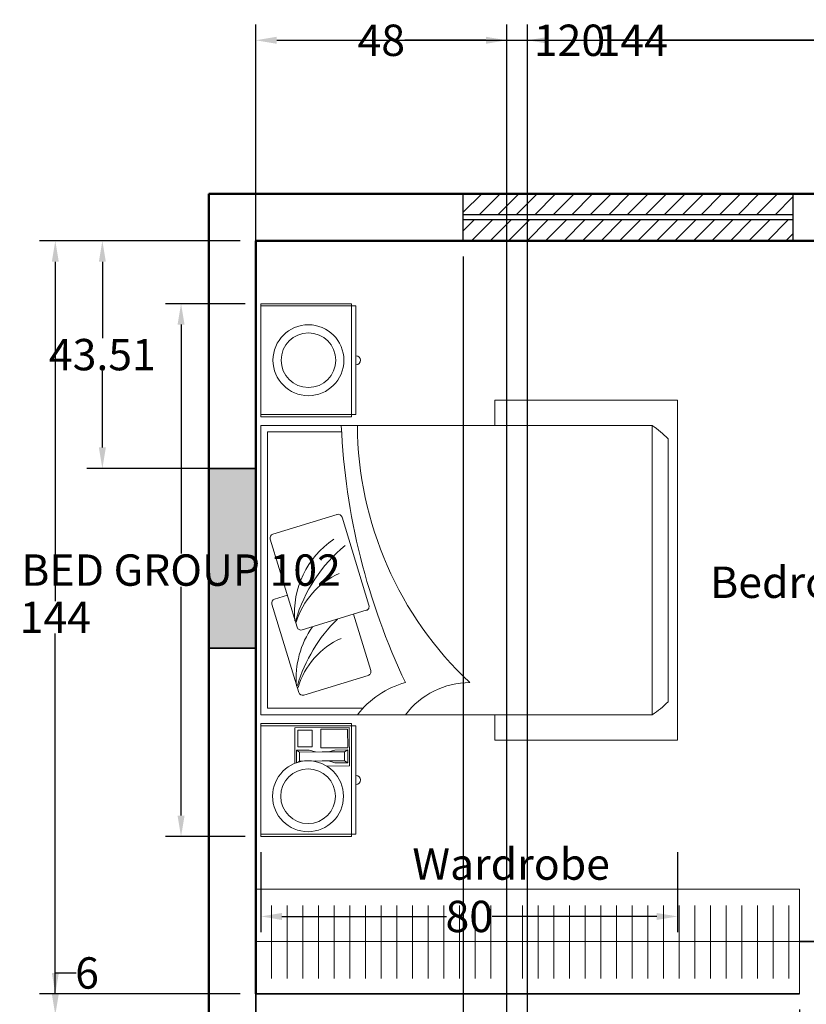
# Model space of a CAD drawing. Units: inches. Extents: x -1285 to -837, y -84 to 552.
# Tile 6 of 10: x -1282 to -1131, y 364 to 552. Entities that reach past the tile are written whole.
import ezdxf

# ---------------------------------------------------------------- set-up
doc = ezdxf.new("R2010")
doc.units = ezdxf.units.IN
doc.header["$MEASUREMENT"] = 0
for name, color, linetype, lineweight in [('A-ANNO-DIMS', 2, 'Continuous', 18), ('A-ANNO-TEXT', 7, 'Continuous', 18), ('A-AREA-IDEN', 7, 'Continuous', 25), ('A-COLS', 54, 'Continuous', 35), ('A-COLS-PATT', 54, 'Continuous', 13), ('A-GLAZ-PATT', 191, 'Continuous', 13), ('Beds', 74, 'Continuous', 18), ('Inner Wall', 202, 'Continuous', 35), ('Outer Wall', 12, 'Continuous', 50), ('Wardrobe', 145, 'Continuous', 18), ('Windows', 191, 'Continuous', 25)]:
    doc.layers.add(name, color=color, linetype=linetype, lineweight=lineweight)
doc.styles.get("Standard").update_dxf_attribs({"font": 'arial.ttf'})
doc.dimstyles.get("Standard").update_dxf_attribs({"dimtxt": 6, "dimasz": 4, "dimexe": 3, "dimexo": 3, "dimgap": 0.09, "dimtad": 0, "dimtih": 1, "dimtoh": 1, "dimdec": 1, "dimzin": 0, "dimdsep": 46, "dimlunit": 3, "dimtxsty": 'Standard', "dimcen": 0.09, "dimadec": 0, "dimazin": 0, "dimtfac": 1, "dimtdec": 1, "dimtofl": 0, "dimtmove": 0, "dimatfit": 3, "dimfxl": 1, "dimtolj": 1, "dimtzin": 0, "dimarcsym": 0})

# ---------------------------------------------------------------- blocks, each defined once
blk = doc.blocks.new('Double bed')
for p, q in [((1422.016, 1006.492), (1422.016, 1015.393)), ((1422.016, 1015.393), (1433.142, 1015.393)), ((1422.239, 1006.047), (1422.239, 1015.393)), ((1432.92, 1015.393), (1432.92, 1006.047)), ((1433.142, 1015.393), (1433.142, 1006.492)), ((1433.999, 1015.393), (1433.999, 1005.908)), ((1462.453, 1015.393), (1433.999, 1015.393)), ((1462.453, 1007.489), (1462.453, 1015.393)), ((1463.309, 1015.393), (1463.309, 1006.491)), ((1474.436, 1015.393), (1463.309, 1015.393)), ((1463.531, 1015.393), (1463.531, 1006.046)), ((1474.214, 1006.046), (1474.214, 1015.393)), ((1474.436, 1006.491), (1474.436, 1015.393)), ((1444.87, 1014.313), (1436.198, 1011.659)), ((1451.273, 1014.487), (1442.6, 1011.833)), ((1451.766, 1014.225), (1453.699, 1007.909)), ((1445.364, 1014.05), (1445.748, 1012.796)), ((1432.723, 1012.072), (1429.217, 1012.059)), ((1429.252, 1011.901), (1430.515, 1011.906)), ((1429.443, 1011.586), (1429.252, 1011.901)), ((1429.443, 1011.586), (1430.327, 1011.589)), ((1429.451, 1009.377), (1429.443, 1011.586)), ((1430.515, 1011.906), (1430.327, 1011.589)), ((1430.335, 1009.38), (1430.327, 1011.589)), ((1430.515, 1011.906), (1430.52, 1010.643)), ((1432.743, 1006.707), (1432.723, 1012.072)), ((1442.338, 1011.34), (1444.27, 1005.024)), ((1430.52, 1010.643), (1430.333, 1010.011)), ((1435.935, 1011.165), (1437.868, 1004.85)), ((1429.411, 1010.132), (1429.449, 1010.008)), ((1429.451, 1009.377), (1429.46, 1007.168)), ((1430.335, 1009.38), (1430.343, 1007.171)), ((1428.948, 1008.926), (1428.957, 1006.693)), ((1429.267, 1008.114), (1429.454, 1008.746)), ((1430.529, 1008.119), (1430.337, 1008.749)), ((1429.272, 1006.852), (1429.267, 1008.114)), ((1430.534, 1006.856), (1430.529, 1008.119)), ((1453.437, 1007.416), (1444.764, 1004.762)), ((1462.453, 1007.489), (1462.453, 976.891)), ((1433.142, 1006.492), (1422.016, 1006.492)), ((1428.957, 1006.693), (1432.743, 1006.707)), ((1429.46, 1007.168), (1429.272, 1006.852)), ((1429.272, 1006.852), (1430.534, 1006.856)), ((1429.46, 1007.168), (1430.343, 1007.171)), ((1430.534, 1006.856), (1430.343, 1007.171)), ((1463.309, 1006.491), (1474.436, 1006.491)), ((1432.92, 1006.047), (1422.239, 1006.047)), ((1433.999, 1005.908), (1433.999, 976.891)), ((1443.887, 1006.278), (1438.362, 1004.587)), ((1463.531, 1006.046), (1474.214, 1006.046)), ((1431.499, 992.391), (1431.499, 974.391)), ((1431.499, 992.391), (1433.999, 992.391)), ((1462.453, 992.391), (1464.953, 992.391)), ((1464.953, 992.391), (1464.953, 974.391)), ((1433.999, 976.891), (1462.453, 976.891)), ((1435.277, 975.333), (1461.153, 975.333)), ((1431.499, 974.391), (1464.953, 974.391))]:
    blk.add_line(p, q)
blk.add_lwpolyline([(1461.821, 1007.458), (1461.821, 1014.761), (1434.631, 1014.761), (1434.631, 1005.368)])
for points in [[(1430.847, 1011.749), (1430.852, 1010.361), (1432.493, 1010.367), (1432.488, 1011.755)], [(1430.745, 1009.508), (1430.755, 1006.857), (1432.585, 1006.864), (1432.575, 1009.515)]]:
    blk.add_lwpolyline(points, close=True)
for points in [[(1433.999, 1005.908, -0.162278), (1437.16, 1001.166, -0.100664), (1462.453, 1007.489, -0.100664)], [(1433.999, 1001.166, -0.236068), (1437.16, 994.843, -0.205258), (1462.453, 1005.908, -0.205258)]]:
    blk.add_lwpolyline(points, format="xyb")
for centre, radius in [((1425.979, 1010.759), 3.489), ((1468.873, 1010.72), 3.49), ((1425.979, 1010.759), 2.689), ((1468.873, 1010.72), 2.688)]:
    blk.add_circle(centre, radius)
for centre, radius, start, end in [((1444.986, 1013.935), 0.395, 17.0142, 107.0142), ((1451.389, 1014.109), 0.395, 17.0142, 107.0142), ((1436.313, 1011.281), 0.395, 107.0142, 197.0142), ((1434.436, 1004.331), 7.75, 24.22087, 73.06906), ((1437.622, 1003.224), 8.697, 54.68511, 95.16051), ((1432.664, 997.407), 14.992, 44.27274, 73.71889), ((1442.716, 1011.455), 0.395, 107.0142, 197.0142), ((1440.838, 1004.506), 7.75, 24.22087, 73.06906), ((1444.025, 1003.399), 8.697, 33.78007, 95.16051), ((1439.066, 997.582), 14.992, 39.40233, 73.71889), ((1453.321, 1007.794), 0.395, 287.0142, 17.0142), ((1427.579, 1006.047), 0.445, 180, 0), ((1468.873, 1006.046), 0.445, 180, 0), ((1438.246, 1004.965), 0.395, 197.0142, 287.0142), ((1444.648, 1005.14), 0.395, 197.0142, 287.0142), ((1441.427, 981.679), 8.838, 212.80295, 225.90033), ((1453.915, 982.69), 10.321, 314.52979, 325.81583)]:
    blk.add_arc(centre, radius, start, end)
blk = doc.blocks.new('Wardrobe')
for p, q in [((958.12, 1084.97), (958.12, 1071.06)), ((961.12, 1084.97), (961.12, 1071.06)), ((964.12, 1084.97), (964.12, 1071.06)), ((967.12, 1084.97), (967.12, 1071.06)), ((970.12, 1084.97), (970.12, 1071.06)), ((973.12, 1084.97), (973.12, 1071.06)), ((976.12, 1084.97), (976.12, 1071.06)), ((979.12, 1084.97), (979.12, 1071.06)), ((982.12, 1084.97), (982.12, 1071.06)), ((985.12, 1084.97), (985.12, 1071.06)), ((988.12, 1084.97), (988.12, 1071.06)), ((991.12, 1084.97), (991.12, 1071.06)), ((994.12, 1084.97), (994.12, 1071.06)), ((997.12, 1084.97), (997.12, 1071.06)), ((1000.12, 1084.97), (1000.12, 1071.06)), ((1003.12, 1084.97), (1003.12, 1071.06)), ((1006.12, 1084.97), (1006.12, 1071.06)), ((1009.12, 1084.97), (1009.12, 1071.06)), ((1012.12, 1084.97), (1012.12, 1071.06)), ((1015.12, 1084.97), (1015.12, 1071.06)), ((1018.12, 1084.97), (1018.12, 1071.06)), ((1021.12, 1084.97), (1021.12, 1071.06)), ((1024.12, 1084.97), (1024.12, 1071.06)), ((1027.12, 1084.97), (1027.12, 1071.06)), ((1030.12, 1084.97), (1030.12, 1071.06)), ((1033.12, 1084.97), (1033.12, 1071.06)), ((1036.12, 1084.97), (1036.12, 1071.06)), ((1039.12, 1084.97), (1039.12, 1071.06)), ((1042.12, 1084.97), (1042.12, 1071.06)), ((1045.12, 1084.97), (1045.12, 1071.06)), ((1048.12, 1084.97), (1048.12, 1071.06)), ((1051.12, 1084.97), (1051.12, 1071.06)), ((1054.12, 1084.97), (1054.12, 1071.06)), ((1057.12, 1084.97), (1057.12, 1071.06)), ((1059.14, 1078.09), (1059.14, 1068.09))]:
    blk.add_line(p, q)
blk.add_lwpolyline([(955.14, 1088.09), (1059.14, 1088.09), (1059.14, 1068.09), (955.14, 1068.09)], close=True)
blk = doc.blocks.new('WIN-63x9')
for p, q in [((4, 63.04), (4, 0)), ((5, 63.04), (5, 0))]:
    blk.add_line(p, q)
blk.add_lwpolyline([(0, 0), (0, 63.04), (9, 63.04), (9, 0)], close=True)
blk = doc.blocks.new('WALL-PIER-34x9')
blk.add_lwpolyline([(9, 34.35), (9, 0), (0, 0), (0, 34.35)], close=True)
blk = doc.blocks.new('*D45')
at = {"layer": 'A-ANNO-DIMS', "color": 0, "lineweight": -2, "transparency": 16777216}
for p, q in [((-1238.55, 497.92), (-1253.83, 497.92)), ((-1250.83, 493.92), (-1250.83, 450.17)), ((-1250.83, 400.03), (-1250.83, 443.78)), ((-1238.55, 396.03), (-1253.83, 396.03))]:
    blk.add_line(p, q, dxfattribs=at)
at = {"layer": 'A-ANNO-DIMS', "color": 0, "transparency": 16777216}
for points in [[(-1251.5, 493.92), (-1250.16, 493.92), (-1250.83, 497.92)], [(-1251.5, 400.03), (-1250.16, 400.03), (-1250.83, 396.03)]]:
    blk.add_solid(points, dxfattribs=at)
at = {"layer": 'Defpoints', "color": 0, "transparency": 16777216}
for p in [(-1250.83, 497.92), (-1235.55, 497.92), (-1235.55, 396.03)]:
    blk.add_point(p, dxfattribs=at)
at = {"layer": 'A-ANNO-DIMS', "color": 0, "transparency": 16777216, "insert": (-1250.83, 446.98), "char_height": 6, "attachment_point": 5}
blk.add_mtext('\\A1;BED GROUP 102', dxfattribs=at)
blk = doc.blocks.new('*D46')
at = {"layer": 'A-ANNO-DIMS', "color": 0, "lineweight": -2, "transparency": 16777216}
for p, q in [((-1235.55, 393.03), (-1235.55, 377.75)), ((-1155.85, 393.03), (-1155.85, 377.75)), ((-1231.55, 380.75), (-1200.08, 380.75)), ((-1159.85, 380.75), (-1191.32, 380.75))]:
    blk.add_line(p, q, dxfattribs=at)
at = {"layer": 'A-ANNO-DIMS', "color": 0, "transparency": 16777216}
for points in [[(-1231.55, 381.41), (-1231.55, 380.08), (-1235.55, 380.75)], [(-1159.85, 381.41), (-1159.85, 380.08), (-1155.85, 380.75)]]:
    blk.add_solid(points, dxfattribs=at)
at = {"layer": 'Defpoints', "color": 0, "transparency": 16777216}
for p in [(-1235.55, 396.03), (-1155.85, 396.03), (-1235.55, 380.75)]:
    blk.add_point(p, dxfattribs=at)
at = {"layer": 'A-ANNO-DIMS', "color": 0, "transparency": 16777216, "insert": (-1195.7, 380.75), "char_height": 6, "attachment_point": 5}
blk.add_mtext('\\A1;80', dxfattribs=at)
blk = doc.blocks.new('*D59')
at = {"layer": 'A-ANNO-DIMS', "color": 0, "lineweight": -2, "transparency": 16777216}
for p, q in [((-1236.53, 362.94), (-1236.53, 347.34)), ((-1132.53, 362.94), (-1132.53, 347.34)), ((-1232.53, 350.34), (-1217.2, 350.34)), ((-1136.53, 350.34), (-1151.86, 350.34))]:
    blk.add_line(p, q, dxfattribs=at)
at = {"layer": 'A-ANNO-DIMS', "color": 0, "transparency": 16777216}
for points in [[(-1232.53, 351.01), (-1232.53, 349.67), (-1236.53, 350.34)], [(-1136.53, 351.01), (-1136.53, 349.67), (-1132.53, 350.34)]]:
    blk.add_solid(points, dxfattribs=at)
at = {"layer": 'Defpoints', "color": 0, "transparency": 16777216}
for p in [(-1236.53, 365.94), (-1132.53, 365.94), (-1132.53, 350.34)]:
    blk.add_point(p, dxfattribs=at)
at = {"layer": 'A-ANNO-DIMS', "color": 0, "transparency": 16777216, "insert": (-1184.53, 350.34), "char_height": 6, "attachment_point": 5}
blk.add_mtext('\\A1;WARDROBE 104', dxfattribs=at)
blk = doc.blocks.new('*D60')
at = {"layer": 'A-ANNO-DIMS', "color": 0, "lineweight": -2, "transparency": 16777216}
for p, q in [((-1129.53, 385.94), (-1113.93, 385.94)), ((-1116.93, 381.94), (-1116.93, 379.09)), ((-1116.93, 369.94), (-1116.93, 372.79)), ((-1129.53, 365.94), (-1113.93, 365.94))]:
    blk.add_line(p, q, dxfattribs=at)
at = {"layer": 'A-ANNO-DIMS', "color": 0, "transparency": 16777216}
for points in [[(-1117.6, 381.94), (-1116.26, 381.94), (-1116.93, 385.94)], [(-1117.6, 369.94), (-1116.26, 369.94), (-1116.93, 365.94)]]:
    blk.add_solid(points, dxfattribs=at)
at = {"layer": 'Defpoints', "color": 0, "transparency": 16777216}
for p in [(-1132.53, 385.94), (-1116.93, 385.94), (-1132.53, 365.94)]:
    blk.add_point(p, dxfattribs=at)
at = {"layer": 'A-ANNO-DIMS', "color": 0, "transparency": 16777216, "insert": (-1116.93, 375.94), "char_height": 6, "attachment_point": 5}
blk.add_mtext('\\A1;20', dxfattribs=at)
blk = doc.blocks.new('*D71')
at = {"layer": 'A-ANNO-DIMS', "color": 0, "lineweight": -2, "transparency": 16777216}
for p, q in [((-1236.53, 512.94), (-1236.53, 551.29)), ((-1092.53, 512.94), (-1092.53, 551.29)), ((-1232.53, 548.29), (-1170.95, 548.29)), ((-1096.53, 548.29), (-1158.11, 548.29))]:
    blk.add_line(p, q, dxfattribs=at)
at = {"layer": 'A-ANNO-DIMS', "color": 0, "transparency": 16777216}
for points in [[(-1232.53, 548.96), (-1232.53, 547.62), (-1236.53, 548.29)], [(-1096.53, 548.96), (-1096.53, 547.62), (-1092.53, 548.29)]]:
    blk.add_solid(points, dxfattribs=at)
at = {"layer": 'Defpoints', "color": 0, "transparency": 16777216}
for p in [(-1092.53, 548.29), (-1236.53, 509.94), (-1092.53, 509.94)]:
    blk.add_point(p, dxfattribs=at)
at = {"layer": 'A-ANNO-DIMS', "color": 0, "transparency": 16777216, "insert": (-1164.53, 548.29), "char_height": 6, "attachment_point": 5}
blk.add_mtext('\\A1;144', dxfattribs=at)
blk = doc.blocks.new('*D74')
at = {"layer": 'A-ANNO-DIMS', "color": 0, "lineweight": -2, "transparency": 16777216}
for p, q in [((-1239.53, 509.94), (-1277.88, 509.94)), ((-1274.88, 505.94), (-1274.88, 441.04)), ((-1274.88, 369.94), (-1274.88, 434.84)), ((-1239.53, 365.94), (-1277.88, 365.94))]:
    blk.add_line(p, q, dxfattribs=at)
at = {"layer": 'A-ANNO-DIMS', "color": 0, "transparency": 16777216}
for points in [[(-1275.55, 505.94), (-1274.21, 505.94), (-1274.88, 509.94)], [(-1275.55, 369.94), (-1274.21, 369.94), (-1274.88, 365.94)]]:
    blk.add_solid(points, dxfattribs=at)
at = {"layer": 'Defpoints', "color": 0, "transparency": 16777216}
for p in [(-1274.88, 509.94), (-1236.53, 509.94), (-1236.53, 365.94)]:
    blk.add_point(p, dxfattribs=at)
at = {"layer": 'A-ANNO-DIMS', "color": 0, "transparency": 16777216, "insert": (-1274.88, 437.94), "char_height": 6, "attachment_point": 5}
blk.add_mtext('\\A1;144', dxfattribs=at)
blk = doc.blocks.new('*D78')
at = {"layer": 'A-ANNO-DIMS', "color": 0, "lineweight": -2, "transparency": 16777216}
for p, q in [((-1236.53, 162.94), (-1236.53, 551.29)), ((-1116.53, 162.94), (-1116.53, 551.29)), ((-1232.53, 548.29), (-1182.96, 548.29)), ((-1120.53, 548.29), (-1170.1, 548.29))]:
    blk.add_line(p, q, dxfattribs=at)
at = {"layer": 'A-ANNO-DIMS', "color": 0, "transparency": 16777216}
for points in [[(-1232.53, 548.96), (-1232.53, 547.62), (-1236.53, 548.29)], [(-1120.53, 548.96), (-1120.53, 547.62), (-1116.53, 548.29)]]:
    blk.add_solid(points, dxfattribs=at)
at = {"layer": 'Defpoints', "color": 0, "transparency": 16777216}
for p in [(-1116.53, 548.29), (-1236.53, 159.94), (-1116.53, 159.94)]:
    blk.add_point(p, dxfattribs=at)
at = {"layer": 'A-ANNO-DIMS', "color": 0, "transparency": 16777216, "insert": (-1176.53, 548.29), "char_height": 6, "attachment_point": 5}
blk.add_mtext('\\A1;120', dxfattribs=at)
blk = doc.blocks.new('*D79')
at = {"layer": 'A-ANNO-DIMS', "color": 0, "lineweight": -2, "transparency": 16777216}
for p, q in [((-1236.53, 38.94), (-1236.53, 551.29)), ((-1188.53, 38.94), (-1188.53, 551.29)), ((-1232.53, 548.29), (-1217.04, 548.29)), ((-1192.53, 548.29), (-1208.02, 548.29))]:
    blk.add_line(p, q, dxfattribs=at)
at = {"layer": 'A-ANNO-DIMS', "color": 0, "transparency": 16777216}
for points in [[(-1232.53, 548.96), (-1232.53, 547.62), (-1236.53, 548.29)], [(-1192.53, 548.96), (-1192.53, 547.62), (-1188.53, 548.29)]]:
    blk.add_solid(points, dxfattribs=at)
at = {"layer": 'Defpoints', "color": 0, "transparency": 16777216}
for p in [(-1188.53, 548.29), (-1236.53, 35.94), (-1188.53, 35.94)]:
    blk.add_point(p, dxfattribs=at)
at = {"layer": 'A-ANNO-DIMS', "color": 0, "transparency": 16777216, "insert": (-1212.53, 548.29), "char_height": 6, "attachment_point": 5}
blk.add_mtext('\\A1;48', dxfattribs=at)
blk = doc.blocks.new('*D80')
at = {"layer": 'A-ANNO-DIMS', "color": 0, "lineweight": -2, "transparency": 16777216}
for p, q in [((-1184.53, -13.66), (-1184.53, 551.29)), ((-1032.53, -13.66), (-1032.53, 551.29)), ((-1180.53, 548.29), (-1114.94, 548.29)), ((-1036.53, 548.29), (-1102.12, 548.29))]:
    blk.add_line(p, q, dxfattribs=at)
at = {"layer": 'A-ANNO-DIMS', "color": 0, "transparency": 16777216}
for points in [[(-1180.53, 548.96), (-1180.53, 547.62), (-1184.53, 548.29)], [(-1036.53, 548.96), (-1036.53, 547.62), (-1032.53, 548.29)]]:
    blk.add_solid(points, dxfattribs=at)
at = {"layer": 'Defpoints', "color": 0, "transparency": 16777216}
for p in [(-1032.53, 548.29), (-1184.53, -16.66), (-1032.53, -16.66)]:
    blk.add_point(p, dxfattribs=at)
at = {"layer": 'A-ANNO-DIMS', "color": 0, "transparency": 16777216, "insert": (-1108.53, 548.29), "char_height": 6, "attachment_point": 5}
blk.add_mtext('\\A1;152', dxfattribs=at)
blk = doc.blocks.new('*D96')
at = {"layer": 'A-ANNO-DIMS', "color": 0, "lineweight": -2, "transparency": 16777216}
for p, q in [((-1236.53, 506.94), (-1236.53, -83.53)), ((-1196.84, 506.94), (-1196.84, -83.53)), ((-1232.53, -80.53), (-1226.9, -80.53)), ((-1200.84, -80.53), (-1206.47, -80.53))]:
    blk.add_line(p, q, dxfattribs=at)
at = {"layer": 'A-ANNO-DIMS', "color": 0, "transparency": 16777216}
for points in [[(-1232.53, -79.86), (-1232.53, -81.2), (-1236.53, -80.53)], [(-1200.84, -79.86), (-1200.84, -81.2), (-1196.84, -80.53)]]:
    blk.add_solid(points, dxfattribs=at)
at = {"layer": 'Defpoints', "color": 0, "transparency": 16777216}
for p in [(-1236.53, 509.94), (-1196.84, 509.94), (-1196.84, -80.53)]:
    blk.add_point(p, dxfattribs=at)
at = {"layer": 'A-ANNO-DIMS', "color": 0, "transparency": 16777216, "insert": (-1216.68, -80.53), "char_height": 6, "attachment_point": 5}
blk.add_mtext('\\A1;39.69', dxfattribs=at)
blk = doc.blocks.new('*D106')
at = {"layer": 'A-ANNO-DIMS', "color": 0, "lineweight": -2, "transparency": 16777216}
for p, q in [((-1274.88, 365.94), (-1274.88, 369.94)), ((-1274.88, 369.94), (-1270.88, 369.94)), ((-983.53, 361.94), (-1277.88, 361.94)), ((-983.53, 355.94), (-1277.88, 355.94)), ((-1274.88, 351.94), (-1274.88, 347.94))]:
    blk.add_line(p, q, dxfattribs=at)
at = {"layer": 'A-ANNO-DIMS', "color": 0, "transparency": 16777216}
for points in [[(-1275.55, 365.94), (-1274.21, 365.94), (-1274.88, 361.94)], [(-1275.55, 351.94), (-1274.21, 351.94), (-1274.88, 355.94)]]:
    blk.add_solid(points, dxfattribs=at)
at = {"layer": 'Defpoints', "color": 0, "transparency": 16777216}
for p in [(-1274.88, 361.94), (-980.53, 361.94), (-980.53, 355.94)]:
    blk.add_point(p, dxfattribs=at)
at = {"layer": 'A-ANNO-DIMS', "color": 0, "transparency": 16777216, "insert": (-1268.81, 369.94), "char_height": 6, "attachment_point": 5}
blk.add_mtext('\\A1;6', dxfattribs=at)
blk = doc.blocks.new('*D111')
at = {"layer": 'A-ANNO-DIMS', "color": 0, "lineweight": -2, "transparency": 16777216}
for p, q in [((-1239.53, 509.94), (-1268.88, 509.94)), ((-1265.88, 505.94), (-1265.88, 491.34)), ((-1265.88, 470.43), (-1265.88, 485.03)), ((-1239.53, 466.43), (-1268.88, 466.43))]:
    blk.add_line(p, q, dxfattribs=at)
at = {"layer": 'A-ANNO-DIMS', "color": 0, "transparency": 16777216}
for points in [[(-1266.55, 505.94), (-1265.21, 505.94), (-1265.88, 509.94)], [(-1266.55, 470.43), (-1265.21, 470.43), (-1265.88, 466.43)]]:
    blk.add_solid(points, dxfattribs=at)
at = {"layer": 'Defpoints', "color": 0, "transparency": 16777216}
for p in [(-1265.88, 509.94), (-1236.53, 509.94), (-1236.53, 466.43)]:
    blk.add_point(p, dxfattribs=at)
at = {"layer": 'A-ANNO-DIMS', "color": 0, "transparency": 16777216, "insert": (-1265.88, 488.18), "char_height": 6, "attachment_point": 5}
blk.add_mtext('\\A1;43.51', dxfattribs=at)

msp = doc.modelspace()

# ---------------------------------------------------------------- hatches: boundary and pattern name
at = {"layer": 'A-COLS-PATT'}
h = msp.add_hatch(color=256, dxfattribs=at)
h.dxf.hatch_style = 1
h.paths.add_polyline_path([(-1236.5299, 354.7957), (-1245.5299, 354.7957), (-1245.5299, 320.4471), (-1236.5299, 320.4471)])
h.paths.add_polyline_path([(-1236.5299, 466.4307), (-1245.5299, 466.4307), (-1245.5299, 432.0821), (-1236.5299, 432.0821)])
h.paths.add_polyline_path([(-877.5299, 151.7586), (-886.5299, 151.7586), (-886.5299, 117.41), (-877.5299, 117.41)])
h.paths.add_polyline_path([(-877.5299, 43.9103), (-886.5299, 43.9103), (-886.5299, -28.0897), (-877.5299, -28.0897)])
h.paths.add_polyline_path([(-1236.5299, 203.7523), (-1245.5299, 203.7523), (-1245.5299, 169.4036), (-1236.5299, 169.4036)])
at = {"layer": 'A-GLAZ-PATT'}
h = msp.add_hatch(dxfattribs=at)
h.set_pattern_fill('ANSI31', color=256, scale=20)
h.set_pattern_definition([(45, (-2191.666, -702.1458), (-1.767767, 1.767767), [])])
h.paths.add_polyline_path([(-921.1945, 518.9392), (-984.2307, 518.9392), (-984.2307, 514.9392), (-921.1945, 514.9392)])
h.paths.add_polyline_path([(-921.1945, 513.9392), (-984.2307, 513.9392), (-984.2307, 509.9392), (-921.1945, 509.9392)])
h.paths.add_polyline_path([(-877.5299, 480.0491), (-881.5299, 480.0491), (-881.5299, 417.0129), (-877.5299, 417.0129)])
h.paths.add_polyline_path([(-882.5299, 480.0491), (-886.5299, 480.0491), (-886.5299, 417.0129), (-882.5299, 417.0129)])
h.paths.add_polyline_path([(-877.5299, 356.1195), (-881.5299, 356.1195), (-881.5299, 321.7709), (-877.5299, 321.7709)])
h.paths.add_polyline_path([(-882.5299, 356.1195), (-886.5299, 356.1195), (-886.5299, 321.7709), (-882.5299, 321.7709)])
h.paths.add_polyline_path([(-1133.8033, 518.9392), (-1196.8396, 518.9392), (-1196.8396, 514.9392), (-1133.8033, 514.9392)])
h.paths.add_polyline_path([(-1133.8033, 513.9392), (-1196.8396, 513.9392), (-1196.8396, 509.9392), (-1133.8033, 509.9392)])
h.paths.add_polyline_path([(-1236.5299, 138.1751), (-1240.5299, 138.1751), (-1240.5299, 75.1388), (-1236.5299, 75.1388)])
h.paths.add_polyline_path([(-1241.5299, 138.1751), (-1245.5299, 138.1751), (-1245.5299, 75.1388), (-1241.5299, 75.1388)])
h.paths.add_polyline_path([(-1236.5299, 35.9392), (-1240.5299, 35.9392), (-1240.5299, 1.5906), (-1236.5299, 1.5906)])
h.paths.add_polyline_path([(-1241.5299, 35.9392), (-1245.5299, 35.9392), (-1245.5299, 1.5906), (-1241.5299, 1.5906)])
h.paths.add_polyline_path([(-1088.8155, -16.6608), (-1136.8155, -16.6608), (-1136.8155, -20.6608), (-1088.8155, -20.6608)])
h.paths.add_polyline_path([(-1088.8155, -21.6608), (-1136.8155, -21.6608), (-1136.8155, -25.6608), (-1088.8155, -25.6608)])

# ---------------------------------------------------------------- linework, layer by layer
at = {"layer": 'Inner Wall'}
for p, q in [((-1132.5299, 375.9392), (-1092.5299, 375.9392)), ((-1236.5299, 365.9392), (-1132.5299, 365.9392))]:
    msp.add_line(p, q, dxfattribs=at)
at = {"layer": 'Outer Wall'}
for p, q in [((-1245.5299, 518.9392), (-877.5299, 518.9392)), ((-1245.5299, 518.9392), (-1245.5299, -51.0608)), ((-1236.5299, 509.9392), (-1236.5299, 365.9392)), ((-1236.5299, 509.9392), (-1092.5299, 509.9392))]:
    msp.add_line(p, q, dxfattribs=at)
at = {"layer": 'Wardrobe'}
msp.add_line((-1132.5299, 375.9392), (-1236.5299, 375.9392), dxfattribs=at)

# ---------------------------------------------------------------- block references
at = {"layer": 'A-COLS'}
msp.add_blockref('WALL-PIER-34x9', (-1245.53, 432.082), dxfattribs=at)
at = {"layer": 'Beds', "xscale": 1.94375808005279, "yscale": 1.94375808005279, "zscale": 1.94375808005279, "rotation": 90}
msp.add_blockref('Double bed', (738.1321, -2368.0247), dxfattribs=at)
at = {"layer": 'Wardrobe'}
msp.add_blockref('Wardrobe', (-2191.666, -702.1458), dxfattribs=at)
at = {"layer": 'Windows', "rotation": 270.0000000000002}
msp.add_blockref('WIN-63x9', (-1196.8394, 518.9394), dxfattribs=at)

# ---------------------------------------------------------------- texts
at = {"layer": 'A-ANNO-TEXT', "insert": (-1206.5742, 393.7648), "char_height": 6, "attachment_point": 1}
msp.add_mtext_dynamic_manual_height_columns('Wardrobe', width=68.784729, gutter_width=1, heights=[0], dxfattribs=at)
at = {"layer": 'A-AREA-IDEN', "insert": (-1149.6203, 447.6499), "char_height": 6, "attachment_point": 1}
msp.add_mtext_dynamic_manual_height_columns('Bedroom 1', width=68.784729, gutter_width=1, heights=[0], dxfattribs=at)

# ---------------------------------------------------------------- dimensions: what is measured, and where the dimension line sits
at = {"layer": 'A-ANNO-DIMS'}
for base, p1, p2, override, picture, middle in [((-1092.5299, 548.2892), (-1236.5299, 509.9392), (-1092.5299, 509.9392), {"dimdec": 0, "dimlfac": 1, "dimrnd": 0, "dimzin": 0, "dimdsep": 46, "dimlunit": 2}, '*D71', (-1164.5299, 548.2892)), ((-1116.5299, 548.2892), (-1236.5299, 159.9392), (-1116.5299, 159.9392), {"dimdec": 0, "dimlfac": 1, "dimrnd": 0, "dimzin": 0, "dimdsep": 46, "dimlunit": 2}, '*D78', (-1176.5299, 548.2892)), ((-1188.5299, 548.2892), (-1236.5299, 35.9392), (-1188.5299, 35.9392), {"dimdec": 0, "dimlfac": 1, "dimrnd": 0, "dimzin": 0, "dimdsep": 46, "dimlunit": 2}, '*D79', (-1212.5299, 548.2892)), ((-1032.5299, 548.2892), (-1184.5299, -16.6608), (-1032.5299, -16.6608), {"dimdec": 0, "dimlfac": 1, "dimrnd": 0, "dimzin": 0, "dimdsep": 46, "dimlunit": 2}, '*D80', (-1108.5299, 548.2892)), ((-1196.8396, -80.5308), (-1236.5299, 509.9392), (-1196.8396, 509.9392), {"dimdec": 2, "dimlfac": 1, "dimrnd": 0, "dimzin": 0, "dimdsep": 46, "dimlunit": 2}, '*D96', (-1216.6847, -80.5308))]:
    dim = msp.add_linear_dim(base=base, p1=p1, p2=p2, dimstyle='Standard', override=override, dxfattribs=at)
    dim.commit()
    dim.dimension.update_dxf_attribs({"geometry": picture, "text_midpoint": middle})
for base, p1, p2, angle, override, picture, middle in [((-1274.8799, 509.9392), (-1236.5299, 365.9392), (-1236.5299, 509.9392), 90, {"dimdec": 0, "dimlfac": 1, "dimrnd": 0, "dimzin": 0, "dimdsep": 46, "dimlunit": 2}, '*D74', (-1274.8799, 437.9392)), ((-1265.8799, 509.9392), (-1236.5299, 466.4307), (-1236.5299, 509.9392), 90, {"dimdec": 2, "dimlfac": 1, "dimrnd": 0, "dimzin": 0, "dimdsep": 46, "dimlunit": 2}, '*D111', (-1265.8799, 488.185)), ((-1235.5466, 380.7473), (-1155.8492, 396.031), (-1235.5466, 396.031), 180, {"dimdec": 0, "dimlfac": 1, "dimrnd": 0, "dimzin": 0, "dimdsep": 46, "dimlunit": 2}, '*D46', (-1195.6979, 380.7473)), ((-1116.9299, 385.9392), (-1132.5299, 365.9392), (-1132.5299, 385.9392), 90, {"dimdec": 0, "dimlfac": 1, "dimrnd": 0, "dimzin": 0, "dimdsep": 46, "dimlunit": 2}, '*D60', (-1116.9299, 375.9392)), ((-1274.8799, 361.9392), (-980.5299, 355.9392), (-980.5299, 361.9392), 90, {"dimdec": 0, "dimlfac": 1, "dimrnd": 0, "dimzin": 0, "dimdsep": 46, "dimlunit": 2}, '*D106', (-1268.809, 369.9392))]:
    dim = msp.add_linear_dim(base=base, p1=p1, p2=p2, angle=angle, dimstyle='Standard', override=override, dxfattribs=at)
    dim.commit()
    dim.dimension.update_dxf_attribs({"geometry": picture, "text_midpoint": middle})
dim = msp.add_linear_dim(base=(-1250.8303, 497.9225), p1=(-1235.5466, 396.031), p2=(-1235.5466, 497.9225), angle=90, text='BED GROUP <>', dimstyle='Standard', override={"dimdec": 0, "dimlfac": 1, "dimrnd": 0, "dimzin": 0, "dimdsep": 46, "dimlunit": 2}, dxfattribs=at)
dim.commit()
dim.dimension.update_dxf_attribs({"geometry": '*D45', "text_midpoint": (-1250.8303, 446.9767)})
dim = msp.add_linear_dim(base=(-1132.5299, 350.3392), p1=(-1236.5299, 365.9392), p2=(-1132.5299, 365.9392), text='WARDROBE <>', dimstyle='Standard', override={"dimdec": 0, "dimlfac": 1, "dimrnd": 0, "dimzin": 0, "dimdsep": 46, "dimlunit": 2}, dxfattribs=at)
dim.commit()
dim.dimension.update_dxf_attribs({"geometry": '*D59', "text_midpoint": (-1184.5299, 350.3392)})

doc.saveas('drawing.dxf')
